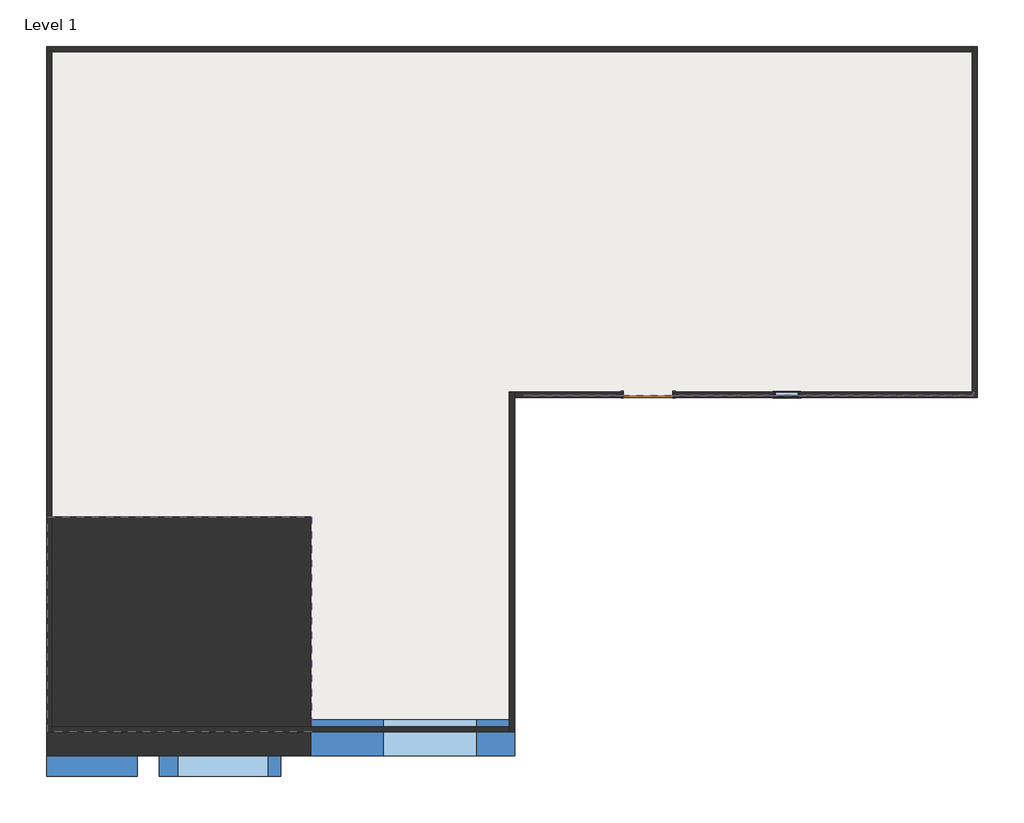
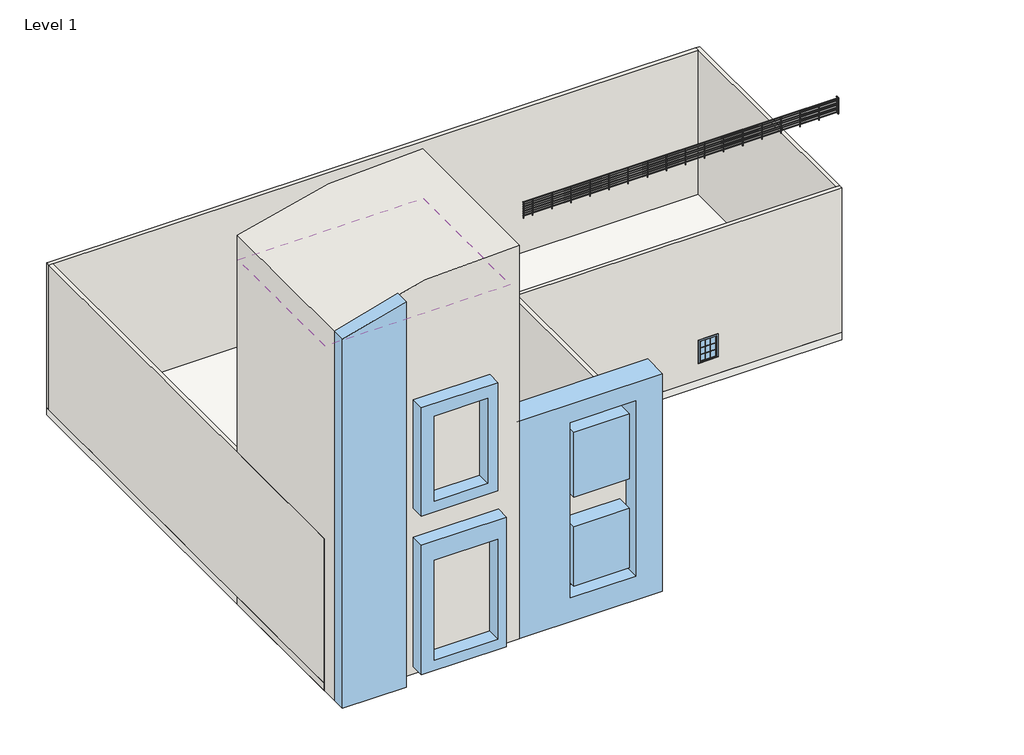
# One storey, part 1 of 2: 7 walls, 3 windows, 1 covering, 1 door, 1 railing, 1 slab.
"""IFC4 building model written with IfcOpenShell, lengths in millimetres."""

from ifc_helpers import new_model, si_unit, point, frame, frame_2d, origin, origin_with_axes, place, context, project, spatial, polyline, circle_curve, ellipse_curve, trimmed, segment, composite_curve, outline, extrude, faceted_brep, transform, mapped, element, save
from ifc_brep_helpers import plane_surface, cylinder_surface, advanced_brep
from components import door_8409b21c, walls_1_walls_1_63333409, window_ddc5d35f, windows_1_windows_1_253e0c66, windows_2_windows_2_da26fb5b

model = new_model("IFC4")

# Units and contexts
model_context = context("Model", 3, world=origin())
ifc_project = project(units=[si_unit("LENGTHUNIT", "METRE", prefix="MILLI")], contexts=[model_context])

# Site, building, storey
site = spatial("IfcSite", under=ifc_project)
building = spatial("IfcBuilding", under=site)
storey = spatial("IfcBuildingStorey", under=building, Name="Level 1", Elevation=0.0)

# Covering
placement = place(None, origin())
element("IfcCovering", 1, ObjectType="600 x 1200mm grid", at=placement, inside=storey, context=model_context, shape_type="SweptSolid", body=[
    extrude(outline(polyline([(-8766.5654563, -9514.7964492), (-18466.5654563, -9514.7964492), (-18466.5654563, -1614.7964492), (-8766.5654563, -1614.7964492), (-8766.5654563, -9514.7964492)])), frame((0.0, 0.0, 18655.0), z_axis=(0.0, 0.0, 1.0), x_axis=(1.0, 0.0, 0.0)), (0.0, 0.0, 1.0), 52.0),
])

# Door
door_shape = door_8409b21c(model_context)
element("IfcDoor", 2, ObjectType="Door-Double-Flush_Panel-Double-Acting : 72\" x 78\"", at=placement, inside=storey, context=model_context, shape_type="MappedRepresentation", body=[
    mapped(door_shape, transform((3597.920453, 2888.3992031, 0.0), x_axis=(-1.0, 0.0, 0.0), y_axis=(0.0, -1.0, 0.0), z_axis=(0.0, 0.0, 1.0))),
])

# Railing
element("IfcRailing", 3, ObjectType="900mm Pipe", at=placement, inside=storey, context=model_context, shape_type="SolidModel", body=[
    advanced_brep(
    [(15526.4612533, 2988.1881175, 12987.4590508), (15566.4612533, 2988.1881175, 12987.4590508), (15526.4612533, 2868.1881175, 12987.4590508), (15566.4612533, 2828.1881175, 12987.4590508), (-953.5387467, 2868.1881175, 12987.4590508), (-953.5387467, 2828.1881175, 12987.4590508)],
    [
        (0, 1, circle_curve(frame((15546.4612533, 2988.1881175, 12987.4590508), z_axis=(0.0, 1.0, 0.0), x_axis=(1.0, 0.0, 0.0)), 20.0)),
        (1, 0, circle_curve(frame((15546.4612533, 2988.1881175, 12987.4590508), z_axis=(0.0, 1.0, 0.0), x_axis=(1.0, 0.0, 0.0)), 20.0)),
        (0, 2),
        (2, 3, ellipse_curve(frame((15546.4612533, 2848.1881175, 12987.4590508), z_axis=(0.7071067811865487, 0.7071067811865464, 0.0), x_axis=(-0.7071067811865464, 0.7071067811865487, 0.0)), 28.2842712, 20.0)),
        (3, 1),
        (3, 2, ellipse_curve(frame((15546.4612533, 2848.1881175, 12987.4590508), z_axis=(0.7071067811865487, 0.7071067811865464, 0.0), x_axis=(-0.7071067811865464, 0.7071067811865487, 0.0)), 28.2842712, 20.0)),
        (4, 5, circle_curve(frame((-953.5387467, 2848.1881175, 12987.4590508), z_axis=(-1.0, 0.0, 0.0), x_axis=(0.0, -1.0, 0.0)), 20.0)),
        (5, 4, circle_curve(frame((-953.5387467, 2848.1881175, 12987.4590508), z_axis=(-1.0, 0.0, 0.0), x_axis=(0.0, -1.0, 0.0)), 20.0)),
        (2, 4),
        (5, 3),
    ],
    [
        plane_surface(frame((15546.4612533, 2988.1881175, 13007.4590508), z_axis=(0.0, 1.0, 0.0), x_axis=(0.0, 0.0, -1.0))),
        cylinder_surface(frame((15546.4612533, 2988.1881175, 12987.4590508), z_axis=(0.0, 1.0, 0.0), x_axis=(1.0, 0.0, 0.0)), 20.0),
        plane_surface(frame((-953.5387467, 2848.1881175, 13007.4590508), z_axis=(-1.0, 0.0, 0.0), x_axis=(0.0, -1.0, 0.0))),
        cylinder_surface(frame((15546.4612533, 2848.1881175, 12987.4590508), z_axis=(1.0, 0.0, 0.0), x_axis=(0.0, -1.0, 0.0)), 20.0),
    ],
    [
        (0, [[1, 2]]),
        (1, [[-1, 3, 4, 5]]),
        (1, [[-2, -5, 6, -3]]),
        (2, [[7, 8]]),
        (3, [[-4, 9, -8, 10]]),
        (3, [[-6, -10, -7, -9]]),
    ],
),
    advanced_brep(
    [(15561.4612533, 2988.1881175, 12867.4590508), (15531.4612533, 2988.1881175, 12867.4590508), (15561.4612533, 2833.1881175, 12867.4590508), (15531.4612533, 2863.1881175, 12867.4590508), (-953.5387467, 2833.1881175, 12867.4590508), (-953.5387467, 2863.1881175, 12867.4590508)],
    [
        (0, 1, circle_curve(frame((15546.4612533, 2988.1881175, 12867.4590508), z_axis=(0.0, 1.0, 0.0), x_axis=(-1.0, 0.0, 0.0)), 15.0)),
        (1, 0, circle_curve(frame((15546.4612533, 2988.1881175, 12867.4590508), z_axis=(0.0, 1.0, 0.0), x_axis=(-1.0, 0.0, 0.0)), 15.0)),
        (0, 2),
        (2, 3, ellipse_curve(frame((15546.4612533, 2848.1881175, 12867.4590508), z_axis=(0.7071067811865487, 0.7071067811865464, 0.0), x_axis=(-0.7071067811865464, 0.7071067811865487, 0.0)), 21.2132034, 15.0)),
        (3, 1),
        (3, 2, ellipse_curve(frame((15546.4612533, 2848.1881175, 12867.4590508), z_axis=(0.7071067811865487, 0.7071067811865464, 0.0), x_axis=(-0.7071067811865464, 0.7071067811865487, 0.0)), 21.2132034, 15.0)),
        (4, 5, circle_curve(frame((-953.5387467, 2848.1881175, 12867.4590508), z_axis=(-1.0, 0.0, 0.0), x_axis=(0.0, 1.0, 0.0)), 15.0)),
        (5, 4, circle_curve(frame((-953.5387467, 2848.1881175, 12867.4590508), z_axis=(-1.0, 0.0, 0.0), x_axis=(0.0, 1.0, 0.0)), 15.0)),
        (2, 4),
        (5, 3),
    ],
    [
        plane_surface(frame((15546.4612533, 2988.1881175, 12882.4590508), z_axis=(0.0, 1.0, 0.0), x_axis=(0.0, 0.0, -1.0))),
        cylinder_surface(frame((15546.4612533, 2988.1881175, 12867.4590508), z_axis=(0.0, 1.0, 0.0), x_axis=(-1.0, 0.0, 0.0)), 15.0),
        plane_surface(frame((-953.5387467, 2848.1881175, 12882.4590508), z_axis=(-1.0, 0.0, 0.0), x_axis=(0.0, -1.0, 0.0))),
        cylinder_surface(frame((15546.4612533, 2848.1881175, 12867.4590508), z_axis=(1.0, 0.0, 0.0), x_axis=(0.0, 1.0, 0.0)), 15.0),
    ],
    [
        (0, [[1, 2]]),
        (1, [[-1, 3, 4, 5]]),
        (1, [[-2, -5, 6, -3]]),
        (2, [[7, 8]]),
        (3, [[-4, 9, -8, 10]]),
        (3, [[-6, -10, -7, -9]]),
    ],
),
    advanced_brep(
    [(15561.4612533, 2988.1881175, 12742.4590508), (15531.4612533, 2988.1881175, 12742.4590508), (15561.4612533, 2833.1881175, 12742.4590508), (15531.4612533, 2863.1881175, 12742.4590508), (-953.5387467, 2833.1881175, 12742.4590508), (-953.5387467, 2863.1881175, 12742.4590508)],
    [
        (0, 1, circle_curve(frame((15546.4612533, 2988.1881175, 12742.4590508), z_axis=(0.0, 1.0, 0.0), x_axis=(-1.0, 0.0, 0.0)), 15.0)),
        (1, 0, circle_curve(frame((15546.4612533, 2988.1881175, 12742.4590508), z_axis=(0.0, 1.0, 0.0), x_axis=(-1.0, 0.0, 0.0)), 15.0)),
        (0, 2),
        (2, 3, ellipse_curve(frame((15546.4612533, 2848.1881175, 12742.4590508), z_axis=(0.7071067811865487, 0.7071067811865464, 0.0), x_axis=(-0.7071067811865464, 0.7071067811865487, 0.0)), 21.2132034, 15.0)),
        (3, 1),
        (3, 2, ellipse_curve(frame((15546.4612533, 2848.1881175, 12742.4590508), z_axis=(0.7071067811865487, 0.7071067811865464, 0.0), x_axis=(-0.7071067811865464, 0.7071067811865487, 0.0)), 21.2132034, 15.0)),
        (4, 5, circle_curve(frame((-953.5387467, 2848.1881175, 12742.4590508), z_axis=(-1.0, 0.0, 0.0), x_axis=(0.0, 1.0, 0.0)), 15.0)),
        (5, 4, circle_curve(frame((-953.5387467, 2848.1881175, 12742.4590508), z_axis=(-1.0, 0.0, 0.0), x_axis=(0.0, 1.0, 0.0)), 15.0)),
        (2, 4),
        (5, 3),
    ],
    [
        plane_surface(frame((15546.4612533, 2988.1881175, 12757.4590508), z_axis=(0.0, 1.0, 0.0), x_axis=(0.0, 0.0, -1.0))),
        cylinder_surface(frame((15546.4612533, 2988.1881175, 12742.4590508), z_axis=(0.0, 1.0, 0.0), x_axis=(-1.0, 0.0, 0.0)), 15.0),
        plane_surface(frame((-953.5387467, 2848.1881175, 12757.4590508), z_axis=(-1.0, 0.0, 0.0), x_axis=(0.0, -1.0, 0.0))),
        cylinder_surface(frame((15546.4612533, 2848.1881175, 12742.4590508), z_axis=(1.0, 0.0, 0.0), x_axis=(0.0, 1.0, 0.0)), 15.0),
    ],
    [
        (0, [[1, 2]]),
        (1, [[-1, 3, 4, 5]]),
        (1, [[-2, -5, 6, -3]]),
        (2, [[7, 8]]),
        (3, [[-4, 9, -8, 10]]),
        (3, [[-6, -10, -7, -9]]),
    ],
),
    advanced_brep(
    [(15561.4612533, 2988.1881175, 12617.4590508), (15531.4612533, 2988.1881175, 12617.4590508), (15561.4612533, 2833.1881175, 12617.4590508), (15531.4612533, 2863.1881175, 12617.4590508), (-953.5387467, 2833.1881175, 12617.4590508), (-953.5387467, 2863.1881175, 12617.4590508)],
    [
        (0, 1, circle_curve(frame((15546.4612533, 2988.1881175, 12617.4590508), z_axis=(0.0, 1.0, 0.0), x_axis=(-1.0, 0.0, 0.0)), 15.0)),
        (1, 0, circle_curve(frame((15546.4612533, 2988.1881175, 12617.4590508), z_axis=(0.0, 1.0, 0.0), x_axis=(-1.0, 0.0, 0.0)), 15.0)),
        (0, 2),
        (2, 3, ellipse_curve(frame((15546.4612533, 2848.1881175, 12617.4590508), z_axis=(0.7071067811865487, 0.7071067811865464, 0.0), x_axis=(-0.7071067811865464, 0.7071067811865487, 0.0)), 21.2132034, 15.0)),
        (3, 1),
        (3, 2, ellipse_curve(frame((15546.4612533, 2848.1881175, 12617.4590508), z_axis=(0.7071067811865487, 0.7071067811865464, 0.0), x_axis=(-0.7071067811865464, 0.7071067811865487, 0.0)), 21.2132034, 15.0)),
        (4, 5, circle_curve(frame((-953.5387467, 2848.1881175, 12617.4590508), z_axis=(-1.0, 0.0, 0.0), x_axis=(0.0, 1.0, 0.0)), 15.0)),
        (5, 4, circle_curve(frame((-953.5387467, 2848.1881175, 12617.4590508), z_axis=(-1.0, 0.0, 0.0), x_axis=(0.0, 1.0, 0.0)), 15.0)),
        (2, 4),
        (5, 3),
    ],
    [
        plane_surface(frame((15546.4612533, 2988.1881175, 12632.4590508), z_axis=(0.0, 1.0, 0.0), x_axis=(0.0, 0.0, -1.0))),
        cylinder_surface(frame((15546.4612533, 2988.1881175, 12617.4590508), z_axis=(0.0, 1.0, 0.0), x_axis=(-1.0, 0.0, 0.0)), 15.0),
        plane_surface(frame((-953.5387467, 2848.1881175, 12632.4590508), z_axis=(-1.0, 0.0, 0.0), x_axis=(0.0, -1.0, 0.0))),
        cylinder_surface(frame((15546.4612533, 2848.1881175, 12617.4590508), z_axis=(1.0, 0.0, 0.0), x_axis=(0.0, 1.0, 0.0)), 15.0),
    ],
    [
        (0, [[1, 2]]),
        (1, [[-1, 3, 4, 5]]),
        (1, [[-2, -5, 6, -3]]),
        (2, [[7, 8]]),
        (3, [[-4, 9, -8, 10]]),
        (3, [[-6, -10, -7, -9]]),
    ],
),
    advanced_brep(
    [(15561.4612533, 2988.1881175, 12492.4590508), (15531.4612533, 2988.1881175, 12492.4590508), (15561.4612533, 2833.1881175, 12492.4590508), (15531.4612533, 2863.1881175, 12492.4590508), (-953.5387467, 2833.1881175, 12492.4590508), (-953.5387467, 2863.1881175, 12492.4590508)],
    [
        (0, 1, circle_curve(frame((15546.4612533, 2988.1881175, 12492.4590508), z_axis=(0.0, 1.0, 0.0), x_axis=(-1.0, 0.0, 0.0)), 15.0)),
        (1, 0, circle_curve(frame((15546.4612533, 2988.1881175, 12492.4590508), z_axis=(0.0, 1.0, 0.0), x_axis=(-1.0, 0.0, 0.0)), 15.0)),
        (0, 2),
        (2, 3, ellipse_curve(frame((15546.4612533, 2848.1881175, 12492.4590508), z_axis=(0.7071067811865487, 0.7071067811865464, 0.0), x_axis=(-0.7071067811865464, 0.7071067811865487, 0.0)), 21.2132034, 15.0)),
        (3, 1),
        (3, 2, ellipse_curve(frame((15546.4612533, 2848.1881175, 12492.4590508), z_axis=(0.7071067811865487, 0.7071067811865464, 0.0), x_axis=(-0.7071067811865464, 0.7071067811865487, 0.0)), 21.2132034, 15.0)),
        (4, 5, circle_curve(frame((-953.5387467, 2848.1881175, 12492.4590508), z_axis=(-1.0, 0.0, 0.0), x_axis=(0.0, 1.0, 0.0)), 15.0)),
        (5, 4, circle_curve(frame((-953.5387467, 2848.1881175, 12492.4590508), z_axis=(-1.0, 0.0, 0.0), x_axis=(0.0, 1.0, 0.0)), 15.0)),
        (2, 4),
        (5, 3),
    ],
    [
        plane_surface(frame((15546.4612533, 2988.1881175, 12507.4590508), z_axis=(0.0, 1.0, 0.0), x_axis=(0.0, 0.0, -1.0))),
        cylinder_surface(frame((15546.4612533, 2988.1881175, 12492.4590508), z_axis=(0.0, 1.0, 0.0), x_axis=(-1.0, 0.0, 0.0)), 15.0),
        plane_surface(frame((-953.5387467, 2848.1881175, 12507.4590508), z_axis=(-1.0, 0.0, 0.0), x_axis=(0.0, -1.0, 0.0))),
        cylinder_surface(frame((15546.4612533, 2848.1881175, 12492.4590508), z_axis=(1.0, 0.0, 0.0), x_axis=(0.0, 1.0, 0.0)), 15.0),
    ],
    [
        (0, [[1, 2]]),
        (1, [[-1, 3, 4, 5]]),
        (1, [[-2, -5, 6, -3]]),
        (2, [[7, 8]]),
        (3, [[-4, 9, -8, 10]]),
        (3, [[-6, -10, -7, -9]]),
    ],
),
    advanced_brep(
    [(15561.4612533, 2988.1881175, 12367.4590508), (15531.4612533, 2988.1881175, 12367.4590508), (15561.4612533, 2833.1881175, 12367.4590508), (15531.4612533, 2863.1881175, 12367.4590508), (-953.5387467, 2833.1881175, 12367.4590508), (-953.5387467, 2863.1881175, 12367.4590508)],
    [
        (0, 1, circle_curve(frame((15546.4612533, 2988.1881175, 12367.4590508), z_axis=(0.0, 1.0, 0.0), x_axis=(-1.0, 0.0, 0.0)), 15.0)),
        (1, 0, circle_curve(frame((15546.4612533, 2988.1881175, 12367.4590508), z_axis=(0.0, 1.0, 0.0), x_axis=(-1.0, 0.0, 0.0)), 15.0)),
        (0, 2),
        (2, 3, ellipse_curve(frame((15546.4612533, 2848.1881175, 12367.4590508), z_axis=(0.7071067811865487, 0.7071067811865464, 0.0), x_axis=(-0.7071067811865464, 0.7071067811865487, 0.0)), 21.2132034, 15.0)),
        (3, 1),
        (3, 2, ellipse_curve(frame((15546.4612533, 2848.1881175, 12367.4590508), z_axis=(0.7071067811865487, 0.7071067811865464, 0.0), x_axis=(-0.7071067811865464, 0.7071067811865487, 0.0)), 21.2132034, 15.0)),
        (4, 5, circle_curve(frame((-953.5387467, 2848.1881175, 12367.4590508), z_axis=(-1.0, 0.0, 0.0), x_axis=(0.0, 1.0, 0.0)), 15.0)),
        (5, 4, circle_curve(frame((-953.5387467, 2848.1881175, 12367.4590508), z_axis=(-1.0, 0.0, 0.0), x_axis=(0.0, 1.0, 0.0)), 15.0)),
        (2, 4),
        (5, 3),
    ],
    [
        plane_surface(frame((15546.4612533, 2988.1881175, 12382.4590508), z_axis=(0.0, 1.0, 0.0), x_axis=(0.0, 0.0, -1.0))),
        cylinder_surface(frame((15546.4612533, 2988.1881175, 12367.4590508), z_axis=(0.0, 1.0, 0.0), x_axis=(-1.0, 0.0, 0.0)), 15.0),
        plane_surface(frame((-953.5387467, 2848.1881175, 12382.4590508), z_axis=(-1.0, 0.0, 0.0), x_axis=(0.0, -1.0, 0.0))),
        cylinder_surface(frame((15546.4612533, 2848.1881175, 12367.4590508), z_axis=(1.0, 0.0, 0.0), x_axis=(0.0, 1.0, 0.0)), 15.0),
    ],
    [
        (0, [[1, 2]]),
        (1, [[-1, 3, 4, 5]]),
        (1, [[-2, -5, 6, -3]]),
        (2, [[7, 8]]),
        (3, [[-4, 9, -8, 10]]),
        (3, [[-6, -10, -7, -9]]),
    ],
),
    advanced_brep(
    [(15561.4612533, 2988.1881175, 12242.4590508), (15531.4612533, 2988.1881175, 12242.4590508), (15561.4612533, 2833.1881175, 12242.4590508), (15531.4612533, 2863.1881175, 12242.4590508), (-953.5387467, 2833.1881175, 12242.4590508), (-953.5387467, 2863.1881175, 12242.4590508)],
    [
        (0, 1, circle_curve(frame((15546.4612533, 2988.1881175, 12242.4590508), z_axis=(0.0, 1.0, 0.0), x_axis=(-1.0, 0.0, 0.0)), 15.0)),
        (1, 0, circle_curve(frame((15546.4612533, 2988.1881175, 12242.4590508), z_axis=(0.0, 1.0, 0.0), x_axis=(-1.0, 0.0, 0.0)), 15.0)),
        (0, 2),
        (2, 3, ellipse_curve(frame((15546.4612533, 2848.1881175, 12242.4590508), z_axis=(0.7071067811865487, 0.7071067811865464, 0.0), x_axis=(-0.7071067811865464, 0.7071067811865487, 0.0)), 21.2132034, 15.0)),
        (3, 1),
        (3, 2, ellipse_curve(frame((15546.4612533, 2848.1881175, 12242.4590508), z_axis=(0.7071067811865487, 0.7071067811865464, 0.0), x_axis=(-0.7071067811865464, 0.7071067811865487, 0.0)), 21.2132034, 15.0)),
        (4, 5, circle_curve(frame((-953.5387467, 2848.1881175, 12242.4590508), z_axis=(-1.0, 0.0, 0.0), x_axis=(0.0, 1.0, 0.0)), 15.0)),
        (5, 4, circle_curve(frame((-953.5387467, 2848.1881175, 12242.4590508), z_axis=(-1.0, 0.0, 0.0), x_axis=(0.0, 1.0, 0.0)), 15.0)),
        (2, 4),
        (5, 3),
    ],
    [
        plane_surface(frame((15546.4612533, 2988.1881175, 12257.4590508), z_axis=(0.0, 1.0, 0.0), x_axis=(0.0, 0.0, -1.0))),
        cylinder_surface(frame((15546.4612533, 2988.1881175, 12242.4590508), z_axis=(0.0, 1.0, 0.0), x_axis=(-1.0, 0.0, 0.0)), 15.0),
        plane_surface(frame((-953.5387467, 2848.1881175, 12257.4590508), z_axis=(-1.0, 0.0, 0.0), x_axis=(0.0, -1.0, 0.0))),
        cylinder_surface(frame((15546.4612533, 2848.1881175, 12242.4590508), z_axis=(1.0, 0.0, 0.0), x_axis=(0.0, 1.0, 0.0)), 15.0),
    ],
    [
        (0, [[1, 2]]),
        (1, [[-1, 3, 4, 5]]),
        (1, [[-2, -5, 6, -3]]),
        (2, [[7, 8]]),
        (3, [[-4, 9, -8, 10]]),
        (3, [[-6, -10, -7, -9]]),
    ],
),
    extrude(outline(composite_curve([segment(trimmed(circle_curve(frame_2d((-453.5387467, 2848.1881175)), 12.5), [point((-453.5387467, 2835.6881175))], [point((-453.5387467, 2860.6881175))], False, "CARTESIAN"), True, "CONTINUOUS"), segment(trimmed(circle_curve(frame_2d((-453.5387467, 2848.1881175)), 12.5), [point((-453.5387467, 2860.6881175))], [point((-453.5387467, 2835.6881175))], False, "CARTESIAN"), True, "CONTINUOUS")], self_intersect=False)), frame((0.0, 0.0, 12107.4590508), z_axis=(0.0, 0.0, 1.0), x_axis=(1.0, 0.0, 0.0)), (0.0, 0.0, 1.0), 860.0),
    extrude(outline(composite_curve([segment(trimmed(circle_curve(frame_2d((546.4612533, 2848.1881175)), 12.5), [point((546.4612533, 2835.6881175))], [point((546.4612533, 2860.6881175))], False, "CARTESIAN"), True, "CONTINUOUS"), segment(trimmed(circle_curve(frame_2d((546.4612533, 2848.1881175)), 12.5), [point((546.4612533, 2860.6881175))], [point((546.4612533, 2835.6881175))], False, "CARTESIAN"), True, "CONTINUOUS")], self_intersect=False)), frame((0.0, 0.0, 12107.4590508), z_axis=(0.0, 0.0, 1.0), x_axis=(1.0, 0.0, 0.0)), (0.0, 0.0, 1.0), 860.0),
    extrude(outline(composite_curve([segment(trimmed(circle_curve(frame_2d((1546.4612533, 2848.1881175)), 12.5), [point((1546.4612533, 2835.6881175))], [point((1546.4612533, 2860.6881175))], False, "CARTESIAN"), True, "CONTINUOUS"), segment(trimmed(circle_curve(frame_2d((1546.4612533, 2848.1881175)), 12.5), [point((1546.4612533, 2860.6881175))], [point((1546.4612533, 2835.6881175))], False, "CARTESIAN"), True, "CONTINUOUS")], self_intersect=False)), frame((0.0, 0.0, 12107.4590508), z_axis=(0.0, 0.0, 1.0), x_axis=(1.0, 0.0, 0.0)), (0.0, 0.0, 1.0), 860.0),
    extrude(outline(composite_curve([segment(trimmed(circle_curve(frame_2d((2546.4612533, 2848.1881175)), 12.5), [point((2546.4612533, 2835.6881175))], [point((2546.4612533, 2860.6881175))], False, "CARTESIAN"), True, "CONTINUOUS"), segment(trimmed(circle_curve(frame_2d((2546.4612533, 2848.1881175)), 12.5), [point((2546.4612533, 2860.6881175))], [point((2546.4612533, 2835.6881175))], False, "CARTESIAN"), True, "CONTINUOUS")], self_intersect=False)), frame((0.0, 0.0, 12107.4590508), z_axis=(0.0, 0.0, 1.0), x_axis=(1.0, 0.0, 0.0)), (0.0, 0.0, 1.0), 860.0),
    extrude(outline(composite_curve([segment(trimmed(circle_curve(frame_2d((3546.4612533, 2848.1881175)), 12.5), [point((3546.4612533, 2835.6881175))], [point((3546.4612533, 2860.6881175))], False, "CARTESIAN"), True, "CONTINUOUS"), segment(trimmed(circle_curve(frame_2d((3546.4612533, 2848.1881175)), 12.5), [point((3546.4612533, 2860.6881175))], [point((3546.4612533, 2835.6881175))], False, "CARTESIAN"), True, "CONTINUOUS")], self_intersect=False)), frame((0.0, 0.0, 12107.4590508), z_axis=(0.0, 0.0, 1.0), x_axis=(1.0, 0.0, 0.0)), (0.0, 0.0, 1.0), 860.0),
    extrude(outline(composite_curve([segment(trimmed(circle_curve(frame_2d((4546.4612533, 2848.1881175)), 12.5), [point((4546.4612533, 2835.6881175))], [point((4546.4612533, 2860.6881175))], False, "CARTESIAN"), True, "CONTINUOUS"), segment(trimmed(circle_curve(frame_2d((4546.4612533, 2848.1881175)), 12.5), [point((4546.4612533, 2860.6881175))], [point((4546.4612533, 2835.6881175))], False, "CARTESIAN"), True, "CONTINUOUS")], self_intersect=False)), frame((0.0, 0.0, 12107.4590508), z_axis=(0.0, 0.0, 1.0), x_axis=(1.0, 0.0, 0.0)), (0.0, 0.0, 1.0), 860.0),
    extrude(outline(composite_curve([segment(trimmed(circle_curve(frame_2d((5546.4612533, 2848.1881175)), 12.5), [point((5546.4612533, 2835.6881175))], [point((5546.4612533, 2860.6881175))], False, "CARTESIAN"), True, "CONTINUOUS"), segment(trimmed(circle_curve(frame_2d((5546.4612533, 2848.1881175)), 12.5), [point((5546.4612533, 2860.6881175))], [point((5546.4612533, 2835.6881175))], False, "CARTESIAN"), True, "CONTINUOUS")], self_intersect=False)), frame((0.0, 0.0, 12107.4590508), z_axis=(0.0, 0.0, 1.0), x_axis=(1.0, 0.0, 0.0)), (0.0, 0.0, 1.0), 860.0),
    extrude(outline(composite_curve([segment(trimmed(circle_curve(frame_2d((6546.4612533, 2848.1881175)), 12.5), [point((6546.4612533, 2835.6881175))], [point((6546.4612533, 2860.6881175))], False, "CARTESIAN"), True, "CONTINUOUS"), segment(trimmed(circle_curve(frame_2d((6546.4612533, 2848.1881175)), 12.5), [point((6546.4612533, 2860.6881175))], [point((6546.4612533, 2835.6881175))], False, "CARTESIAN"), True, "CONTINUOUS")], self_intersect=False)), frame((0.0, 0.0, 12107.4590508), z_axis=(0.0, 0.0, 1.0), x_axis=(1.0, 0.0, 0.0)), (0.0, 0.0, 1.0), 860.0),
    extrude(outline(composite_curve([segment(trimmed(circle_curve(frame_2d((7546.4612533, 2848.1881175)), 12.5), [point((7546.4612533, 2835.6881175))], [point((7546.4612533, 2860.6881175))], False, "CARTESIAN"), True, "CONTINUOUS"), segment(trimmed(circle_curve(frame_2d((7546.4612533, 2848.1881175)), 12.5), [point((7546.4612533, 2860.6881175))], [point((7546.4612533, 2835.6881175))], False, "CARTESIAN"), True, "CONTINUOUS")], self_intersect=False)), frame((0.0, 0.0, 12107.4590508), z_axis=(0.0, 0.0, 1.0), x_axis=(1.0, 0.0, 0.0)), (0.0, 0.0, 1.0), 860.0),
    extrude(outline(composite_curve([segment(trimmed(circle_curve(frame_2d((8546.4612533, 2848.1881175)), 12.5), [point((8546.4612533, 2835.6881175))], [point((8546.4612533, 2860.6881175))], False, "CARTESIAN"), True, "CONTINUOUS"), segment(trimmed(circle_curve(frame_2d((8546.4612533, 2848.1881175)), 12.5), [point((8546.4612533, 2860.6881175))], [point((8546.4612533, 2835.6881175))], False, "CARTESIAN"), True, "CONTINUOUS")], self_intersect=False)), frame((0.0, 0.0, 12107.4590508), z_axis=(0.0, 0.0, 1.0), x_axis=(1.0, 0.0, 0.0)), (0.0, 0.0, 1.0), 860.0),
    extrude(outline(composite_curve([segment(trimmed(circle_curve(frame_2d((9546.4612533, 2848.1881175)), 12.5), [point((9546.4612533, 2835.6881175))], [point((9546.4612533, 2860.6881175))], False, "CARTESIAN"), True, "CONTINUOUS"), segment(trimmed(circle_curve(frame_2d((9546.4612533, 2848.1881175)), 12.5), [point((9546.4612533, 2860.6881175))], [point((9546.4612533, 2835.6881175))], False, "CARTESIAN"), True, "CONTINUOUS")], self_intersect=False)), frame((0.0, 0.0, 12107.4590508), z_axis=(0.0, 0.0, 1.0), x_axis=(1.0, 0.0, 0.0)), (0.0, 0.0, 1.0), 860.0),
    extrude(outline(composite_curve([segment(trimmed(circle_curve(frame_2d((10546.4612533, 2848.1881175)), 12.5), [point((10546.4612533, 2835.6881175))], [point((10546.4612533, 2860.6881175))], False, "CARTESIAN"), True, "CONTINUOUS"), segment(trimmed(circle_curve(frame_2d((10546.4612533, 2848.1881175)), 12.5), [point((10546.4612533, 2860.6881175))], [point((10546.4612533, 2835.6881175))], False, "CARTESIAN"), True, "CONTINUOUS")], self_intersect=False)), frame((0.0, 0.0, 12107.4590508), z_axis=(0.0, 0.0, 1.0), x_axis=(1.0, 0.0, 0.0)), (0.0, 0.0, 1.0), 860.0),
    extrude(outline(composite_curve([segment(trimmed(circle_curve(frame_2d((11546.4612533, 2848.1881175)), 12.5), [point((11546.4612533, 2835.6881175))], [point((11546.4612533, 2860.6881175))], False, "CARTESIAN"), True, "CONTINUOUS"), segment(trimmed(circle_curve(frame_2d((11546.4612533, 2848.1881175)), 12.5), [point((11546.4612533, 2860.6881175))], [point((11546.4612533, 2835.6881175))], False, "CARTESIAN"), True, "CONTINUOUS")], self_intersect=False)), frame((0.0, 0.0, 12107.4590508), z_axis=(0.0, 0.0, 1.0), x_axis=(1.0, 0.0, 0.0)), (0.0, 0.0, 1.0), 860.0),
    extrude(outline(composite_curve([segment(trimmed(circle_curve(frame_2d((12546.4612533, 2848.1881175)), 12.5), [point((12546.4612533, 2835.6881175))], [point((12546.4612533, 2860.6881175))], False, "CARTESIAN"), True, "CONTINUOUS"), segment(trimmed(circle_curve(frame_2d((12546.4612533, 2848.1881175)), 12.5), [point((12546.4612533, 2860.6881175))], [point((12546.4612533, 2835.6881175))], False, "CARTESIAN"), True, "CONTINUOUS")], self_intersect=False)), frame((0.0, 0.0, 12107.4590508), z_axis=(0.0, 0.0, 1.0), x_axis=(1.0, 0.0, 0.0)), (0.0, 0.0, 1.0), 860.0),
    extrude(outline(composite_curve([segment(trimmed(circle_curve(frame_2d((13546.4612533, 2848.1881175)), 12.5), [point((13546.4612533, 2835.6881175))], [point((13546.4612533, 2860.6881175))], False, "CARTESIAN"), True, "CONTINUOUS"), segment(trimmed(circle_curve(frame_2d((13546.4612533, 2848.1881175)), 12.5), [point((13546.4612533, 2860.6881175))], [point((13546.4612533, 2835.6881175))], False, "CARTESIAN"), True, "CONTINUOUS")], self_intersect=False)), frame((0.0, 0.0, 12107.4590508), z_axis=(0.0, 0.0, 1.0), x_axis=(1.0, 0.0, 0.0)), (0.0, 0.0, 1.0), 860.0),
    extrude(outline(composite_curve([segment(trimmed(circle_curve(frame_2d((14546.4612533, 2848.1881175)), 12.5), [point((14546.4612533, 2835.6881175))], [point((14546.4612533, 2860.6881175))], False, "CARTESIAN"), True, "CONTINUOUS"), segment(trimmed(circle_curve(frame_2d((14546.4612533, 2848.1881175)), 12.5), [point((14546.4612533, 2860.6881175))], [point((14546.4612533, 2835.6881175))], False, "CARTESIAN"), True, "CONTINUOUS")], self_intersect=False)), frame((0.0, 0.0, 12107.4590508), z_axis=(0.0, 0.0, 1.0), x_axis=(1.0, 0.0, 0.0)), (0.0, 0.0, 1.0), 860.0),
    extrude(outline(composite_curve([segment(trimmed(circle_curve(frame_2d((15546.4612533, 2848.1881175)), 12.5), [point((15558.9612533, 2848.1881175))], [point((15533.9612533, 2848.1881175))], False, "CARTESIAN"), True, "CONTINUOUS"), segment(trimmed(circle_curve(frame_2d((15546.4612533, 2848.1881175)), 12.5), [point((15533.9612533, 2848.1881175))], [point((15558.9612533, 2848.1881175))], False, "CARTESIAN"), True, "CONTINUOUS")], self_intersect=False)), frame((0.0, 0.0, 12107.4590508), z_axis=(0.0, 0.0, 1.0), x_axis=(1.0, 0.0, 0.0)), (0.0, 0.0, 1.0), 860.0),
    extrude(outline(composite_curve([segment(trimmed(circle_curve(frame_2d((-941.0387467, 2848.1881175)), 12.5), [point((-941.0387467, 2835.6881175))], [point((-941.0387467, 2860.6881175))], False, "CARTESIAN"), True, "CONTINUOUS"), segment(trimmed(circle_curve(frame_2d((-941.0387467, 2848.1881175)), 12.5), [point((-941.0387467, 2860.6881175))], [point((-941.0387467, 2835.6881175))], False, "CARTESIAN"), True, "CONTINUOUS")], self_intersect=False)), frame((0.0, 0.0, 12107.4590508), z_axis=(0.0, 0.0, 1.0), x_axis=(1.0, 0.0, 0.0)), (0.0, 0.0, 1.0), 860.0),
    extrude(outline(composite_curve([segment(trimmed(circle_curve(frame_2d((15546.4612533, 2975.6881175)), 12.5), [point((15558.9612533, 2975.6881175))], [point((15533.9612533, 2975.6881175))], False, "CARTESIAN"), True, "CONTINUOUS"), segment(trimmed(circle_curve(frame_2d((15546.4612533, 2975.6881175)), 12.5), [point((15533.9612533, 2975.6881175))], [point((15558.9612533, 2975.6881175))], False, "CARTESIAN"), True, "CONTINUOUS")], self_intersect=False)), frame((0.0, 0.0, 12107.4590508), z_axis=(0.0, 0.0, 1.0), x_axis=(1.0, 0.0, 0.0)), (0.0, 0.0, 1.0), 860.0),
])

# Slab
element("IfcSlab", 4, ObjectType="Generic Floor - 400mm", at=placement, inside=storey, context=model_context, shape_type="SweptSolid", body=[
    extrude(outline(polyline([(15697.920453, 15683.5992031), (15697.920453, 2788.3992031), (-1302.079547, 2788.3992031), (-1302.079547, -9516.4007969), (-18502.079547, -9516.4007969), (-18502.079547, 15683.5992031), (15697.920453, 15683.5992031)])), frame((0.0, 0.0, -400.0), z_axis=(0.0, 0.0, 1.0), x_axis=(1.0, 0.0, 0.0)), (0.0, 0.0, 1.0), 400.0),
])

# Walls
element("IfcWall", 5, ObjectType="Generic - 200mm", at=placement, inside=storey, context=model_context, shape_type="Brep", body=[
    faceted_brep([(-18502.079547, 15483.5992031, 8000.0), (-18502.079547, 15483.5992031, 4000.0), (-18502.079547, 15483.5992031, 0.0), (-18302.079547, 15483.5992031, 0.0), (15497.920453, 15483.5992031, 0.0), (15497.920453, 15483.5992031, 8000.0), (-18302.079547, 15483.5992031, 8000.0), (-18502.079547, 15683.5992031, 0.0), (-18502.079547, 15683.5992031, 8000.0), (-18302.079547, 15683.5992031, 8000.0), (15497.920453, 15683.5992031, 8000.0), (15497.920453, 15683.5992031, 0.0)], [[[0, 1, 2, 3, 4, 5, 6]], [[7, 8, 9, 10, 11]], [[4, 3, 2, 7, 11]], [[0, 6, 5, 10, 9, 8]], [[0, 8, 7, 2, 1]], [[4, 11, 10, 5]]]),
])
element("IfcWall", 6, ObjectType="Generic - 200mm", at=placement, inside=storey, context=model_context, shape_type="Brep", body=[
    faceted_brep([(-18302.079547, -9516.4007969, 8000.0), (-18302.079547, -9516.4007969, 4000.0), (-18302.079547, -9516.4007969, 0.0), (-18302.079547, -9316.4007969, 0.0), (-18302.079547, 15483.5992031, 0.0), (-18302.079547, 15483.5992031, 8000.0), (-18302.079547, -9316.4007969, 8000.0), (-18502.079547, -9516.4007969, 0.0), (-18502.079547, -9516.4007969, 8000.0), (-18502.079547, -9316.4007969, 8000.0), (-18502.079547, 15483.5992031, 8000.0), (-18502.079547, 15483.5992031, 0.0)], [[[0, 1, 2, 3, 4, 5, 6]], [[7, 8, 9, 10, 11]], [[4, 3, 2, 7, 11]], [[0, 6, 5, 10, 9, 8]], [[0, 8, 7, 2, 1]], [[4, 11, 10, 5]]]),
])
element("IfcWall", 7, ObjectType="Generic - 200mm", at=placement, inside=storey, context=model_context, shape_type="SweptSolid", body=[
    extrude(outline(polyline([(-18302.079547, -9316.4007969), (-1502.079547, -9316.4007969), (-1502.079547, -9516.4007969), (-18302.079547, -9516.4007969), (-18302.079547, -9316.4007969)])), origin_with_axes(), (0.0, 0.0, 1.0), 8000.0),
])
element("IfcWall", 8, ObjectType="Generic - 200mm", at=placement, inside=storey, context=model_context, shape_type="Brep", body=[
    faceted_brep([(15497.920453, 15683.5992031, 8000.0), (15497.920453, 15683.5992031, 4000.0), (15497.920453, 15683.5992031, 0.0), (15497.920453, 15483.5992031, 0.0), (15497.920453, 2988.3992031, 0.0), (15497.920453, 2988.3992031, 8000.0), (15497.920453, 15483.5992031, 8000.0), (15697.920453, 15683.5992031, 0.0), (15697.920453, 15683.5992031, 8000.0), (15697.920453, 15483.5992031, 8000.0), (15697.920453, 2988.3992031, 8000.0), (15697.920453, 2988.3992031, 0.0)], [[[0, 1, 2, 3, 4, 5, 6]], [[7, 8, 9, 10, 11]], [[4, 3, 2, 7, 11]], [[0, 6, 5, 10, 9, 8]], [[0, 8, 7, 2, 1]], [[4, 11, 10, 5]]]),
])
element("IfcWall", 9, ObjectType="Generic - 200mm", at=placement, inside=storey, context=model_context, shape_type="Brep", body=[
    faceted_brep([(-1302.079547, -9516.4007969, 8000.0), (-1302.079547, -9516.4007969, 0.0), (-1302.079547, 2788.3992031, 0.0), (-1302.079547, 2988.3992031, 0.0), (-1302.079547, 2988.3992031, 4000.0), (-1302.079547, 2988.3992031, 8000.0), (-1302.079547, 2788.3992031, 8000.0), (-1302.079547, -9316.4007969, 8000.0), (-1502.079547, -9516.4007969, 0.0), (-1502.079547, -9516.4007969, 4000.0), (-1502.079547, -9516.4007969, 8000.0), (-1502.079547, -9316.4007969, 8000.0), (-1502.079547, 2788.3992031, 8000.0), (-1502.079547, 2988.3992031, 8000.0), (-1502.079547, 2988.3992031, 0.0), (-1502.079547, -9316.4007969, 0.0)], [[[0, 1, 2, 3, 4, 5, 6, 7]], [[8, 9, 10, 11, 12, 13, 14, 15]], [[3, 2, 1, 8, 15, 14]], [[0, 7, 6, 5, 13, 12, 11, 10]], [[3, 14, 13, 5, 4]], [[0, 10, 9, 8, 1]]]),
])
element("IfcWall", 10, ObjectType="Generic - 200mm", at=placement, inside=storey, context=model_context, shape_type="Brep", body=[
    faceted_brep([(15697.920453, 2788.3992031, 8000.0), (15497.920453, 2788.3992031, 8000.0), (-1302.079547, 2788.3992031, 8000.0), (-1302.079547, 2788.3992031, 0.0), (2683.520453, 2788.3992031, 0.0), (2683.520453, 2788.3992031, 1981.2), (4512.320453, 2788.3992031, 1981.2), (4512.320453, 2788.3992031, 0.0), (15697.920453, 2788.3992031, 0.0), (8240.720453, 2788.3992031, 2133.6), (9155.120453, 2788.3992031, 2133.6), (9155.120453, 2788.3992031, 914.4), (8240.720453, 2788.3992031, 914.4), (-1302.079547, 2988.3992031, 8000.0), (15497.920453, 2988.3992031, 8000.0), (15697.920453, 2988.3992031, 8000.0), (15697.920453, 2988.3992031, 4000.0), (15697.920453, 2988.3992031, 0.0), (15497.920453, 2988.3992031, 0.0), (4512.320453, 2988.3992031, 0.0), (4512.320453, 2988.3992031, 1981.2), (2683.520453, 2988.3992031, 1981.2), (2683.520453, 2988.3992031, 0.0), (-1302.079547, 2988.3992031, 0.0), (8240.720453, 2988.3992031, 2133.6), (8240.720453, 2988.3992031, 914.4), (9155.120453, 2988.3992031, 914.4), (9155.120453, 2988.3992031, 2133.6)], [[[0, 1, 2, 3, 4, 5, 6, 7, 8], [9, 10, 11, 12]], [[13, 14, 15, 16, 17, 18, 19, 20, 21, 22, 23], [24, 25, 26, 27]], [[3, 23, 22, 4]], [[17, 8, 7, 19, 18]], [[2, 1, 0, 15, 14, 13]], [[8, 17, 16, 15, 0]], [[2, 13, 23, 3]], [[21, 5, 4, 22]], [[5, 21, 20, 6]], [[6, 20, 19, 7]], [[25, 24, 9, 12]], [[26, 25, 12, 11]], [[27, 26, 11, 10]], [[24, 27, 10, 9]]]),
])
walls_1_walls_1_shape = walls_1_walls_1_63333409(model_context)
element("IfcWall", 11, ObjectType="Walls 1 : Walls 1", at=placement, inside=storey, context=model_context, shape_type="MappedRepresentation", body=[
    mapped(walls_1_walls_1_shape, transform((0.0, 0.0, 0.0), x_axis=(1.0, 0.0, 0.0), y_axis=(0.0, 1.0, 0.0), z_axis=(0.0, 0.0, 1.0))),
])

# Windows
window_shape = window_ddc5d35f(model_context)
element("IfcWindow", 12, ObjectType="Casement 3x3 with Trim : 36\" x 48\"", at=placement, inside=storey, context=model_context, shape_type="MappedRepresentation", body=[
    mapped(window_shape, transform((8697.920453, 2888.3992031, 0.0), x_axis=(-1.0, 0.0, 0.0), y_axis=(0.0, -1.0, 0.0), z_axis=(0.0, 0.0, 1.0))),
])
windows_1_windows_1_shape = windows_1_windows_1_253e0c66(model_context)
element("IfcWindow", 13, ObjectType="Windows 1 : Windows 1", at=placement, inside=storey, context=model_context, shape_type="MappedRepresentation", body=[
    mapped(windows_1_windows_1_shape, transform((0.0, 0.0, 0.0), x_axis=(1.0, 0.0, 0.0), y_axis=(0.0, 1.0, 0.0), z_axis=(0.0, 0.0, 1.0))),
])
windows_2_windows_2_shape = windows_2_windows_2_da26fb5b(model_context)
element("IfcWindow", 14, ObjectType="Windows 2 : Windows 2", at=placement, inside=storey, context=model_context, shape_type="MappedRepresentation", body=[
    mapped(windows_2_windows_2_shape, transform((0.0, 0.0, 0.0), x_axis=(1.0, 0.0, 0.0), y_axis=(0.0, 1.0, 0.0), z_axis=(0.0, 0.0, 1.0))),
])

save(model, "model.ifc")

# Revit data of these elements
# Type "600 x 1200mm grid"
#   built-in parameter 1002203 = 1 (stored number, unit not read)
#   built-in parameter 1002202 = 1 (stored number, unit not read)
#   Layers, outside or top first: 0' - 1.41732" "Default" (function 1); 0' - 0.62992" "Ceiling Tile 600 x 1200" (function 5)
# Type "Door-Double-Flush_Panel-Double-Acting : 72\" x 78\""
#   Type Mark = "22"
#   Construction Type Id = "DOOR"
#   Assembly Code = "C1020"
#   Analytic Construction = "Wooden"
#   W = 3' - 0"
#   Thickness = 0' - 2"
#   Thermal Resistance (R) = 0.455703 (m²·K)/W
#   Swing Angle [instance default] = 90.00°
#   Heat Transfer Coefficient (U) = 2.19465 W/(m²·K)
#   Height = 6' - 6"
#   Trim Projection Ext. = 0' - 1"
#   Trim Projection Int. = 0' - 1"
#   Trim Width Ext. = 0' - 3"
#   Trim Width Int. = 0' - 3"
#   Width = 6' - 0"
#   Define Thermal Properties by = 1
#   Panel Material = Wood - Birch - Solid Stained Light Low Gloss
#   Trim Material = Paint - Sienna
#   Visual Light Transmittance = 0
#   Solar Heat Gain Coefficient = 0
#   Function = (empty or 0)
#   Wall Closure = (empty or 0)
# Type "900mm Pipe"
#   built-in parameter 1008612 = 0.019685 (stored number, unit not read)
#   built-in parameter 1008611 = 0.0984252 (stored number, unit not read)
#   built-in parameter 1008609 = 6.56168 (stored number, unit not read)
#   built-in parameter 1008604 = 0.19685 (stored number, unit not read)
#   built-in parameter 1008603 = 0.164042 (stored number, unit not read)
#   Railing Height = 2' - 11.43307"
#   built-in parameter 1008630 = 2
#   built-in parameter 1008610 = 2
#   built-in parameter 1008605 = 1
#   built-in parameter 1008618 = M_Baluster - Round : 25mm
# Type "Generic Floor - 400mm"
#   Function = 0
#   Layers, outside or top first: 1' - 3.74803" no material (function 1)
# Type "Generic - 200mm"
#   Layers, outside or top first: 0' - 7.87402" no material (function 1)
# Type "Casement 3x3 with Trim : 36\" x 48\""
#   Type Mark = "19"
#   Construction Type Id = "GSP4R"
#   Assembly Code = "B2020100"
#   Analytic Construction = "1/8 in Pilkington single glazing"
#   Visual Light Transmittance = 0.9
#   Solar Heat Gain Coefficient = 0.78
#   Heat Transfer Coefficient (U) = 3.6886 W/(m²·K)
#   Height = 4' - 0"
#   Default Sill Height = 3' - 0"
#   Trim Projection - Ext. = 0' - 0 1/2"
#   Trim Projection - Int. = 0' - 0 3/4"
#   Trim Width - Exterior = 0' - 3 1/2"
#   Trim Width - Interior = 0' - 3 1/2"
#   Width = 3' - 0"
#   Window Inset = 0' - 0 3/4"
#   Define Thermal Properties by = 1
#   Glass Pane Material = Glass
#   Sash Material = Sash
#   Trim Exterior Material = Trim
#   Trim Interior Material = Trim
#   Wall Closure = (empty or 0)
# Type "Windows 1 : Windows 1"
#   Type Mark = "24"
# Type "Windows 2 : Windows 2"
#   Type Mark = "23"
# Element 1 (IfcCovering, "600 x 1200mm grid")
#   Height Offset From Level = 61' - 2.44882"
#   Phase Created = New Construction
#   Materials on its faces: "Ceiling Tile 600 x 1200", "Default"
# Element 2 (IfcDoor, "Door-Double-Flush_Panel-Double-Acting : 72\" x 78\"")
#   Swing Angle = 90.00°
#   Phase Created = New Construction
#   Materials on its faces: "Paint - Sienna", "Wood - Birch - Solid Stained Light Low Gloss"
# Element 3 (IfcRailing, "900mm Pipe")
#   built-in parameter 1008621 = 39.7226 (stored number, unit not read)
#   Phase Created = New Construction
# Element 4 (IfcSlab, "Generic Floor - 400mm")
#   Height Offset From Level = 0' - 0"
#   Phase Created = New Construction
#   Materials on its faces: "Default Roof"
# Elements 5, 6, 7, 8, 9, 10 (IfcWall, "Generic - 200mm")
#   Top Offset = 0' - 0"
#   Base Offset = 0' - 0"
#   Unconnected Height = 26' - 2.96063"
#   wall height = 26' - 2.96063"
#   Phase Created = New Construction
#   Base Constraint = Level 1
#   Materials on its faces: "Default Wall"
# Element 11 (IfcWall, "Walls 1 : Walls 1")
#   Phase Created = New Construction
#   Materials on its faces: "Default Wall"
# Element 12 (IfcWindow, "Casement 3x3 with Trim : 36\" x 48\"")
#   Mark = "6"
#   Phase Created = New Construction
#   Materials on its faces: "Sash", "Glass", "Trim"
# Element 13 (IfcWindow, "Windows 1 : Windows 1")
#   Mark = "14"
#   Phase Created = New Construction
# Element 14 (IfcWindow, "Windows 2 : Windows 2")
#   Mark = "13"
#   Phase Created = New Construction
# Materials
#   "Default": colour RGB 80 80 80, transparency 0
#   "Ceiling Tile 600 x 1200": class "Generic", colour RGB 179 178 175, transparency 0, Description = "Acoustic ceiling tile", Cost = 0
#   "Wood - Birch - Solid Stained Light Low Gloss": class "Wood", colour RGB 210 159 95, transparency 0, Cost = 0
#   "Paint - Sienna": colour RGB 118 70 51, transparency 0, Cost = 0
#   "Glass": class "Glass", colour RGB 218 227 224, transparency 0.85, Description = "Soda Lime Glass", Cost = 0
#   "Sash": class "Wood", colour RGB 136 99 55, transparency 0
#   "Trim": class "Wood", colour RGB 224 178 126, transparency 0
#   "Default Roof": colour RGB 80 80 80, transparency 0
#   "Default Wall": colour RGB 80 80 80, transparency 0
